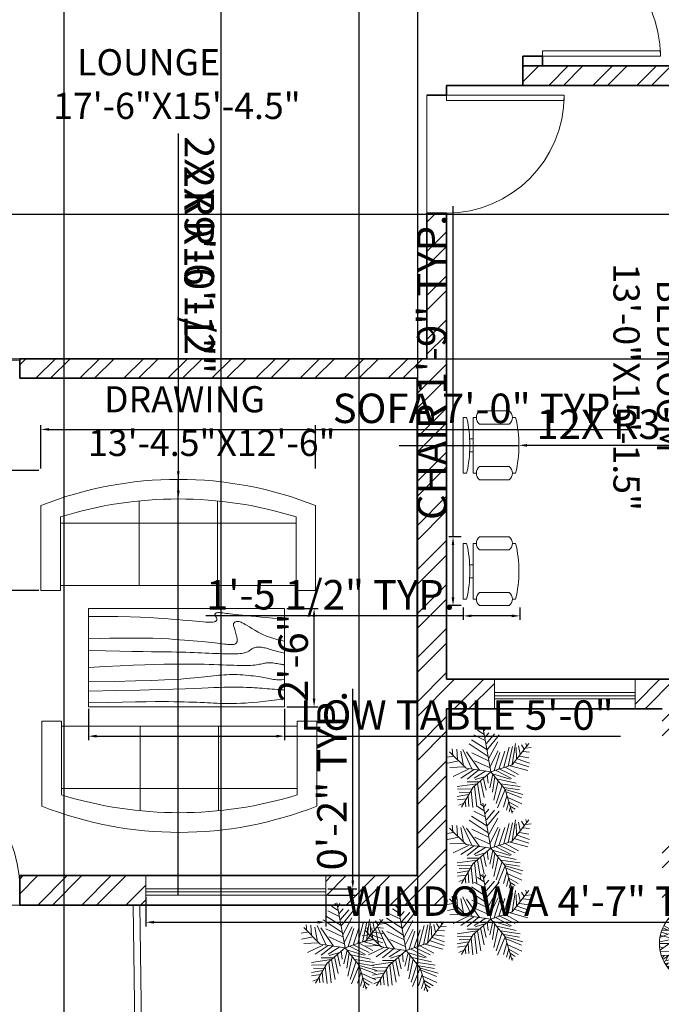
# Model space of a CAD drawing. Units: inches. Extents: x 744 to 1448, y 5126 to 6077.
# Tile 3 of 10: x 1025 to 1221, y 5284 to 5585. Entities that reach past the tile are written whole.
import ezdxf

# ---------------------------------------------------------------- set-up
doc = ezdxf.new("R2010")
doc.units = ezdxf.units.IN
for name, color, linetype, lineweight in [('A-ANNO-DIMS', 2, 'Continuous', 18), ('A-AREA-IDEN', 7, 'Continuous', 18), ('A-DOOR', 4, 'Continuous', 18), ('A-FURN', 8, 'Continuous', 18), ('A-SITE-PVMT', 8, 'Continuous', 18), ('A-WALL', 7, 'Continuous', 35), ('A-WALL-PATT', 252, 'Continuous', 13), ('L-PLNT', 3, 'Continuous', 13)]:
    doc.layers.add(name, color=color, linetype=linetype, lineweight=lineweight)
doc.layers.add('A-GLAZ', color=244, linetype='Continuous', lineweight=18, true_color=0x991b1e)
doc.styles.get("Standard").update_dxf_attribs({"font": 'arial.ttf'})
doc.dimstyles.new('ISO-25', dxfattribs={"dimtxt": 9, "dimasz": 2.5, "dimexe": 1.25, "dimexo": 0.625, "dimtad": 1, "dimlunit": 3, "dimtxsty": 'Standard', "dimcen": 2.5, "dimadec": 0, "dimazin": 0, "dimtfac": 1, "dimtmove": 0, "dimatfit": 3, "dimfxl": 1, "dimarcsym": 0})

# ---------------------------------------------------------------- blocks, each defined once
blk = doc.blocks.new('*U2')
for p, q in [((0, 0), (0, -6)), ((40, 0), (40, -6))]:
    blk.add_line(p, q)
blk.add_lwpolyline([(0, 0), (0, 40), (1.75, 40), (1.75, 0)], close=True)
blk.add_arc((0, 0), 40, 0, 90)
blk = doc.blocks.new('*U5')
for p, q in [((0, 0), (0, 6)), ((40, 0), (40, 6))]:
    blk.add_line(p, q)
blk.add_lwpolyline([(0, 0), (0, -40), (1.75, -40), (1.75, 0)], close=True)
blk.add_arc((0, 0), 40, 270, 0)
blk = doc.blocks.new('*U3')
for p, q in [((-40, 0), (-40, 6)), ((0, 0), (0, 6))]:
    blk.add_line(p, q)
blk.add_lwpolyline([(0, 0), (0, -40), (-1.75, -40), (-1.75, 0)], close=True)
blk.add_arc((0, 0), 40, 180, 270)
blk = doc.blocks.new('*U10')
for p, q in [((-8.737, 47.138), (-17.069, 52.711)), ((-10.186, 53.64), (-13.084, 55.962)), ((0, 0), (-10.5, 57)), ((-9.099, 51.782), (-6.563, 55.962)), ((-5.114, 28.097), (-24.676, 40.636)), ((-7.288, 39.707), (-21.778, 46.673)), ((-7.65, 43.423), (-2.578, 49.46)), ((-5.839, 35.992), (4.667, 48.067)), ((-5.114, 27.632), (10.463, 46.673)), ((-2.941, 16.486), (8.652, 37.85)), ((-31.5, 4.5), (-52.5, 25.5)), ((-48.585, 21.131), (-49.309, 29.026)), ((-43.513, 28.561), (-42.427, 15.558)), ((-38.442, 26.239), (-34.819, 7.663)), ((-35.544, 28.097), (-24.314, 3.947)), ((-14.533, 2.09), (-30.834, 25.31)), ((-3.665, 19.273), (-27.574, 35.527)), ((-1.129, 6.734), (9.014, 26.704)), ((10.101, 3.483), (17.708, 26.239)), ((16.259, 5.805), (23.142, 31.348)), ((22.055, 7.198), (27.489, 32.277)), ((27, 9), (48, 36)), ((27.127, 9.056), (31.112, 35.992)), ((31.836, 30.883), (32.561, 16.486)), ((35.096, 32.741), (37.27, 22.524)), ((38.719, 34.134), (41.979, 28.561)), ((40.53, 25.775), (48.862, 24.846)), ((43.791, 29.954), (51.036, 30.883)), ((44.153, 36.456), (45.239, 32.741)), ((-47.498, 19.737), (-55.83, 18.344)), ((-40.615, 13.7), (-55.105, 10.913)), ((-24.314, 23.917), (-2.941, 13.7)), ((-20.691, 13.7), (-1.129, 4.876)), ((3.942, 1.625), (11.187, 24.381)), ((33.285, 16.486), (48.862, 10.913)), ((36.183, 19.737), (48.137, 17.88)), ((-33.37, 6.269), (-52.207, 5.34)), ((-28.299, 3.483), (-47.86, -5.805)), ((-21.416, 3.018), (-38.079, -8.128)), ((0, 0), (-31.5, 4.5)), ((-15.982, 2.09), (-30.11, -9.521)), ((0, 0), (-22.5, -19.5)), ((-6.563, 1.161), (-21.416, -8.128)), ((0, 0), (27, 9)), ((0, 0), (18, -22.5)), ((6.478, 1.625), (26.04, -8.592)), ((11.187, 3.483), (30.749, -5.805)), ((18.07, 5.805), (35.096, -3.483)), ((24.229, 7.663), (46.688, 1.625)), ((29.662, 12.307), (48.137, 6.269)), ((-6.563, -5.805), (-19.967, -9.985)), ((-13.446, -11.378), (-8.737, -32.741)), ((-9.461, -8.592), (-6.201, -23.453)), ((-4.752, -3.483), (-3.665, -14.629)), ((2.493, -3.019), (-1.491, -20.202)), ((1.769, -2.555), (24.229, -9.521)), ((5.029, -6.27), (2.131, -25.775)), ((9.014, -11.378), (3.58, -35.992)), ((7.565, -9.056), (32.198, -14.629)), ((-17.431, -15.094), (-42.789, -18.809)), ((-24.314, -21.596), (-42.427, -22.06)), ((-22.5, -19.5), (-37.5, -45)), ((-15.257, -12.772), (-30.11, -12.772)), ((-25.038, -23.918), (-22.865, -45.281)), ((-20.691, -18.345), (-17.793, -44.352)), ((-17.069, -15.094), (-12.721, -40.172)), ((14.085, -16.951), (6.478, -40.172)), ((18.07, -22.524), (8.289, -45.745)), ((12.274, -15.094), (36.907, -18.809)), ((16.259, -19.738), (36.183, -22.989)), ((18, -22.5), (27, -52.5)), ((18.433, -22.524), (40.53, -29.026)), ((-28.299, -29.026), (-42.789, -31.348)), ((-30.834, -34.135), (-42.427, -35.528)), ((-26.849, -26.24), (-40.253, -25.775)), ((-32.646, -36.921), (-31.921, -44.352)), ((-29.023, -30.884), (-27.936, -43.887)), ((20.244, -30.419), (15.897, -44.816)), ((19.157, -25.311), (38.719, -33.206)), ((21.331, -32.741), (39.081, -40.636)), ((-34.457, -39.708), (-40.978, -42.494)), ((22.78, -37.85), (19.519, -48.532)), ((22.78, -38.314), (34.372, -44.816)), ((24.591, -45.745), (23.142, -50.854)), ((24.591, -43.423), (30.749, -47.603)), ((26.764, -49.925), (28.213, -50.854))]:
    blk.add_line(p, q)
blk = doc.blocks.new('*U13')
for p, q in [((-37.0107, 47.0408), (-35.25, 35.5298)), ((-32.6092, 50.4264), (-23.2782, 23.5674)), ((-31.2008, 51.1035), (-0.2149, 20.1818)), ((-26.4472, 46.5894), (-26.2712, 53.8116)), ((-22.0458, 42.0753), (-16.5881, 57.6486)), ((-21.1656, 55.8436), (-0.0388, 45.0094)), ((-12.5388, 54.9406), (-7.9613, 59.4546)), ((-12.3627, 32.1443), (-12.5388, 58.7776)), ((-5.3205, 59.6806), (16.5105, 16.7963)), ((2.426, 54.9406), (-1.4472, 59.9056)), ((0, 59.9996), (0, -60)), ((0.4894, 48.6208), (3.6584, 59.6806)), ((18.2711, 35.5298), (5.419, 59.6806)), ((9.8203, 51.5549), (12.8133, 58.5516)), ((19.6795, 19.5047), (16.3344, 57.6486)), ((17.0387, 51.1035), (23.2006, 55.1666)), ((17.7429, 43.6552), (25.4894, 54.2636)), ((31.6513, 50.8778), (30.2429, 30.5643)), ((31.1232, 42.5267), (35.8767, 48.1693)), ((-49.8627, 32.8214), (-32.7853, 32.8214)), ((-45.8134, 38.2383), (-40.5318, 33.0471)), ((-43.8768, 36.4326), (-44.405, 40.2696)), ((42, 42), (-42, -42)), ((42, -42), (-42, 42)), ((-40.1797, 44.558), (-36.4825, 43.2038)), ((36.2288, 25.1474), (48.9049, 35.0784)), ((37.1091, 37.1098), (46.6161, 37.5612)), ((-32.2571, 20.6333), (-59.1937, 9.348)), ((-57.081, 17.9248), (-47.0458, 14.7649)), ((-56.0247, 20.859), (-20.8134, 20.859)), ((-54.7923, 24.4702), (-47.75, 21.0847)), ((-53.2078, 27.4044), (-40.1797, 20.859)), ((54.3626, 25.3731), (20.9119, 0.3198)), ((23.3767, 23.3417), (53.3063, 27.4044)), ((-59.7219, 2.8025), (-12.0106, 12.0565)), ((-58.6656, 12.7336), (-35.9543, 7.5424)), ((-54.6162, -24.7335), (-20.2853, 0.0941)), ((29.3626, -6.6771), (59.4682, 7.091)), ((38.5175, 13.4107), (58.2359, 13.6364)), ((-60, 0), (60, 0)), ((-59.7219, -4.8714), (-54.2641, -6.6771)), ((-45.2853, -0.1316), (-59.0177, -10.0627)), ((-58.4895, -12.3197), (-36.4825, -11.6426)), ((-14.8275, -15.0282), (-14.6515, -57.6865)), ((-10.074, -10.0627), (-2.5036, -59.7178)), ((9.2922, -9.1598), (59.6443, -2.8401)), ((26.3697, -18.4138), (58.9401, -9.8369)), ((-57.081, -18.4138), (-45.2853, -17.9624)), ((-52.6797, -18.188), (-55.4966, -22.0251)), ((-53.2078, -27.442), (-16.7641, -16.6081)), ((-38.9472, -29.0219), (-51.4472, -30.6018)), ((-47.2219, -19.3166), (-50.2148, -26.3135)), ((-46.5177, -30.1504), (-49.5106, -33.536)), ((-35.9543, -22.4765), (-44.0529, -40.5329)), ((-19.9331, -20.2194), (-28.5599, -52.721)), ((-0.0388, -19.0909), (25.8415, -53.8495)), ((18.6232, -18.6394), (26.7218, -53.3981)), ((18.7992, -18.6394), (57.3556, -17.2853)), ((30.419, -30.1504), (32.3556, -50.0125)), ((38.1654, -18.188), (52.426, -29.0219)), ((45.9119, -24.0564), (55.595, -22.2508)), ((-32.4331, -32.4075), (-48.1021, -35.5674)), ((-43.7008, -34.6645), (-46.6937, -37.373)), ((-24.6867, -37.8244), (-38.7712, -45.7241)), ((-26.2712, -43.9185), (-34.7219, -48.6583)), ((-14.6515, -36.2445), (-27.6797, -52.9467)), ((-21.5177, -45.4984), (-19.9331, -56.1065)), ((-14.6515, -32.1818), (-3.912, -59.4922)), ((-6.2008, -36.2445), (17.919, -57.0094)), ((22.8485, -36.4702), (35.3485, -48.4326)), ((24.7852, -44.8213), (23.0246, -54.978)), ((31.4753, -31.279), (49.6091, -33.3103)), ((41.5105, -32.6332), (46.088, -38.0501)), ((-14.6515, -47.3041), (-25.0388, -54.3009)), ((-8.4895, -47.5298), (-11.4825, -58.5893)), ((-6.3768, -52.721), (-9.3698, -58.815)), ((8.4119, -53.1724), (3.8344, -59.4922)), ((5.9471, -46.6269), (10.5246, -58.5893))]:
    blk.add_line(p, q)
blk.add_circle((0, 0), 60)
blk = doc.blocks.new('Table - Rectangular Woodgrain 60 x 30 in.')
for p, q in [((0, 0), (0, -30)), ((60, 0), (0, 0)), ((60, -30), (60, 0)), ((0, -30), (60, -30))]:
    blk.add_line(p, q)
for points in [[(0, -2.4), (4.8155, -2.418), (9.0302, -2.4688), (12.709, -2.5477), (15.9167, -2.65), (18.7181, -2.7711), (21.1781, -2.9063), (23.3616, -3.0508), (25.3333, -3.2), (27.1477, -3.3495), (28.8172, -3.4958), (30.3437, -3.636), (31.7291, -3.7667), (32.9756, -3.8849), (34.0849, -3.9875), (35.059, -4.0714), (35.9, -4.1334), (36.6114, -4.1711), (37.2041, -4.1854), (37.6906, -4.1779), (38.0833, -4.15), (38.3948, -4.1034), (38.6375, -4.0396), (38.8239, -3.9602), (38.9666, -3.8667), (39.0764, -3.7608), (39.1573, -3.6448), (39.2116, -3.521), (39.2416, -3.3917), (39.2498, -3.2593), (39.2385, -3.1261), (39.21, -2.9944), (39.1666, -2.8667), (39.111, -2.7447), (39.0468, -2.6281), (38.978, -2.5163), (38.9083, -2.4083), (38.8418, -2.3035), (38.7823, -2.201), (38.7337, -2.1001), (38.7, -2), (38.6844, -1.9003), (38.6875, -1.8021), (38.7094, -1.707), (38.75, -1.6167), (38.8094, -1.5326), (38.8875, -1.4563), (38.9844, -1.3893), (39.1, -1.3333), (39.2351, -1.2896), (39.3937, -1.2583), (39.5804, -1.2396), (39.8, -1.2333), (40.057, -1.2396), (40.3562, -1.2583), (40.7023, -1.2896), (41.1, -1.3333), (41.5547, -1.3895), (42.0755, -1.4573), (42.6721, -1.5361), (43.3542, -1.625), (44.1316, -1.7233), (45.014, -1.8302), (46.0114, -1.9449), (47.1333, -2.0667), (48.3862, -2.1947), (49.7625, -2.3281), (51.2513, -2.4663), (52.8416, -2.6083), (54.5226, -2.7535), (56.2833, -2.9011), (58.1127, -3.0501), (60, -3.2)], [(0, -9.2), (6.5759, -9.0858), (11.9385, -9.0365), (16.2527, -9.0418), (19.6833, -9.0917), (22.3952, -9.1759), (24.5531, -9.2844), (26.322, -9.4069), (27.8666, -9.5333), (29.3241, -9.6553), (30.7203, -9.7719), (32.0532, -9.8837), (33.3208, -9.9917), (34.5213, -10.0965), (35.6526, -10.199), (36.7128, -10.2999), (37.7, -10.4), (38.6129, -10.4996), (39.4531, -10.5969), (40.223, -10.6895), (40.925, -10.775), (41.5613, -10.8512), (42.1344, -10.9156), (42.6465, -10.966), (43.1, -11), (43.4976, -11.0158), (43.8437, -11.0136), (44.143, -10.9942), (44.4, -10.9583), (44.6195, -10.9069), (44.8062, -10.8406), (44.9648, -10.7603), (45.1, -10.6667), (45.2155, -10.5598), (45.3114, -10.4365), (45.3871, -10.2929), (45.4416, -10.125), (45.4743, -9.929), (45.4844, -9.7011), (45.4709, -9.4371), (45.4333, -9.1333), (45.3716, -8.7883), (45.2896, -8.4104), (45.1919, -8.0107), (45.0833, -7.6), (44.9685, -7.1893), (44.8521, -6.7896), (44.7388, -6.4117), (44.6333, -6.0667), (44.54, -5.7628), (44.4614, -5.4979), (44.4001, -5.2675), (44.3583, -5.0667), (44.3384, -4.8909), (44.3427, -4.7354), (44.3736, -4.5956), (44.4333, -4.4667), (44.5236, -4.3453), (44.6427, -4.2333), (44.7884, -4.1339), (44.9583, -4.05), (45.1501, -3.9849), (45.3614, -3.9417), (45.59, -3.9234), (45.8333, -3.9333), (46.0915, -3.9749), (46.3734, -4.0531), (46.6906, -4.1736), (47.0542, -4.3417), (47.4756, -4.5629), (47.9661, -4.8427), (48.5372, -5.1866), (49.2, -5.6), (49.9676, -6.0844), (50.8594, -6.625), (51.8965, -7.2031), (53.1, -7.8), (54.491, -8.3969), (56.0906, -8.975), (57.9199, -9.5156), (60, -10)], [(0, -12.8), (5.1847, -12.9322), (9.6213, -13.0323), (13.3963, -13.1059), (16.5958, -13.1583), (19.3063, -13.1952), (21.614, -13.2219), (23.6054, -13.2439), (25.3666, -13.2667), (26.9728, -13.2947), (28.4531, -13.3281), (29.8256, -13.3663), (31.1083, -13.4083), (32.3191, -13.4535), (33.476, -13.501), (34.597, -13.5501), (35.7, -13.6), (36.7984, -13.6497), (37.8875, -13.6979), (38.9578, -13.743), (40, -13.7833), (41.0047, -13.8174), (41.9625, -13.8438), (42.864, -13.8607), (43.7, -13.8667), (44.4631, -13.8604), (45.1552, -13.8417), (45.7801, -13.8104), (46.3416, -13.7667), (46.8439, -13.7104), (47.2906, -13.6417), (47.6858, -13.5604), (48.0333, -13.4667), (48.3375, -13.3608), (48.6042, -13.2448), (48.8396, -13.121), (49.05, -12.9917), (49.2417, -12.8593), (49.4208, -12.7261), (49.5937, -12.5944), (49.7667, -12.4667), (49.9452, -12.3451), (50.1323, -12.2313), (50.3303, -12.1268), (50.5416, -12.0333), (50.7686, -11.9524), (51.0135, -11.8854), (51.2788, -11.8341), (51.5666, -11.8), (51.8785, -11.7843), (52.2116, -11.7865), (52.562, -11.8059), (52.926, -11.8417), (53.2998, -11.8931), (53.6795, -11.9594), (54.0614, -12.0397), (54.4416, -12.1333), (54.8223, -12.2401), (55.2293, -12.3625), (55.6942, -12.5037), (56.2489, -12.6667), (56.9251, -12.8547), (57.7545, -13.0708), (58.7689, -13.3182), (60, -13.6)], [(0, -18), (5.124, -17.7273), (9.6609, -17.5057), (13.6705, -17.3303), (17.2125, -17.1958), (20.3467, -17.0973), (23.1328, -17.0297), (25.6307, -16.9878), (27.9, -16.9667), (29.9928, -16.9617), (31.9302, -16.9703), (33.7254, -16.9907), (35.3917, -17.0208), (36.9423, -17.0588), (38.3906, -17.1026), (39.7499, -17.1503), (41.0333, -17.2), (42.2519, -17.2496), (43.4073, -17.2969), (44.4986, -17.3395), (45.525, -17.375), (46.4858, -17.4012), (47.3802, -17.4156), (48.2074, -17.416), (48.9667, -17.4), (49.6583, -17.3662), (50.2872, -17.3167), (50.8595, -17.2547), (51.3812, -17.1833), (51.8584, -17.1057), (52.2971, -17.025), (52.7034, -16.9443), (53.0833, -16.8667), (53.443, -16.7951), (53.789, -16.7313), (54.128, -16.6768), (54.4666, -16.6334), (54.8115, -16.6024), (55.1693, -16.5854), (55.5465, -16.5841), (55.95, -16.6), (56.3828, -16.6337), (56.8346, -16.6823), (57.2915, -16.7418), (57.7396, -16.8084), (58.165, -16.878), (58.5539, -16.9469), (58.8924, -17.0111), (59.1666, -17.0667), (59.3679, -17.1107), (59.5078, -17.1438), (59.6032, -17.1675), (59.6708, -17.1833), (59.7275, -17.193), (59.7901, -17.1979), (59.8753, -17.1998), (60, -17.2)], [(0, -22.4), (8.0098, -22.2501), (14.4094, -22.1011), (19.4168, -21.9535), (23.25, -21.8083), (26.1269, -21.6663), (28.2656, -21.5281), (29.884, -21.3947), (31.2, -21.2667), (32.3967, -21.1448), (33.5172, -21.0292), (34.5697, -20.9198), (35.5625, -20.8167), (36.5037, -20.7198), (37.4015, -20.6292), (38.2642, -20.5448), (39.1, -20.4667), (39.9164, -20.3951), (40.7187, -20.3313), (41.5117, -20.2768), (42.3, -20.2333), (43.0883, -20.2024), (43.8812, -20.1854), (44.6836, -20.1841), (45.5, -20.2), (46.3328, -20.234), (47.1747, -20.2844), (48.0163, -20.3488), (48.8479, -20.425), (49.66, -20.5106), (50.4429, -20.6031), (51.1872, -20.7004), (51.8833, -20.8), (52.5246, -20.8999), (53.1166, -20.9995), (53.6681, -21.0983), (54.1875, -21.1958), (54.6834, -21.2919), (55.1646, -21.3859), (55.6394, -21.4777), (56.1167, -21.5667), (56.6028, -21.6515), (57.0961, -21.7266), (57.5929, -21.7852), (58.0896, -21.8208), (58.5823, -21.8268), (59.0674, -21.7964), (59.5412, -21.723), (60, -21.6)], [(0, -25.2), (8.6355, -25.0504), (15.7026, -24.9031), (21.4049, -24.7606), (25.9458, -24.625), (29.529, -24.4988), (32.3578, -24.3844), (34.6359, -24.284), (36.5667, -24.2), (38.3213, -24.1341), (39.9417, -24.0854), (41.437, -24.0523), (42.8167, -24.0333), (44.0901, -24.0268), (45.2667, -24.0313), (46.3557, -24.0451), (47.3667, -24.0667), (48.309, -24.0947), (49.1928, -24.1287), (50.0284, -24.168), (50.826, -24.2125), (51.5959, -24.2617), (52.3483, -24.3151), (53.0935, -24.3725), (53.8417, -24.4334), (54.6009, -24.497), (55.3699, -24.561), (56.1454, -24.6226), (56.9239, -24.6792), (57.7021, -24.7279), (58.4764, -24.7662), (59.2435, -24.7911), (60, -24.8)], [(0, -28.8), (5.6867, -28.6681), (10.45, -28.5698), (14.407, -28.5012), (17.675, -28.4584), (20.3711, -28.4374), (22.6125, -28.4344), (24.5164, -28.4455), (26.2, -28.4667), (27.762, -28.4947), (29.2276, -28.5281), (30.6033, -28.5663), (31.8958, -28.6084), (33.1118, -28.6535), (34.2578, -28.7011), (35.3405, -28.7501), (36.3666, -28.8), (37.3443, -28.8497), (38.288, -28.8974), (39.2137, -28.9412), (40.1375, -28.9792), (41.0753, -29.0093), (42.0432, -29.0297), (43.0572, -29.0384), (44.1333, -29.0333), (45.2936, -29.0114), (46.5843, -28.9641), (48.0579, -28.8816), (49.7666, -28.7542), (51.7629, -28.5721), (54.0989, -28.3255), (56.8272, -28.0048), (60, -27.6)]]:
    blk.add_lwpolyline(points)
blk = doc.blocks.new('Sofa - Roundback 7 ft.')
for p, q in [((-12.00002, -32.4421), (-12.00003, -6.5971)), ((11.99997, -32.4421), (11.99998, -6.5971)), ((-36.000027, -34), (-36.000027, -11.4696)), ((35.99998, -34), (35.99998, -11.4696)), ((-35.999844, -13.3819), (35.9998, -13.3819)), ((-36.000027, -32.4421), (35.99998, -32.4421))]:
    blk.add_line(p, q)
for points in [[(-36.000027, -34), (-42.000027, -34), (-42.000027, -8)], [(41.99998, -8), (41.99998, -34), (35.99998, -34)]]:
    blk.add_lwpolyline(points)
for centre, radius, start, end in [((0, -114.25), 114.25, 68.43141, 111.5686), ((-0.00001, -127.1968), 121.1968, 72.72033, 107.2797)]:
    blk.add_arc(centre, radius, start, end)
blk = doc.blocks.new('Chair - Desk')
for p, q in [((-8.5, 0), (-8.5, -1)), ((-8.5, 0), (8.5, 0)), ((8.5, 0), (8.5, -1)), ((-8.5, -3), (-8.5, -4)), ((-8.5, -3), (8.5, -3)), ((-2, -3), (-2, -1.9355)), ((2, -1.9576), (2, -3)), ((8.5, -3), (8.5, -4)), ((-10.5, -5), (-10.5, -14)), ((-6.5, -14), (-6.5, -5)), ((6.5, -5), (6.5, -14)), ((10.5, -14), (10.5, -5)), ((-8.5, -15), (-8.5, -16)), ((8.5, -15), (8.5, -16))]:
    blk.add_line(p, q)
for centre, radius, start, end in [((0, 34.625), 36.625, 256.5803, 283.4197), ((-8.5, -6.5), 2.5, 36.8699, 143.1301), ((8.5, -6.5), 2.5, 36.8699, 143.1301), ((-8.5, -12.5), 2.5, 216.8699, 323.1301), ((8.5, -12.5), 2.5, 216.8699, 323.1301), ((0, 19.625), 36.625, 256.5803, 283.4197)]:
    blk.add_arc(centre, radius, start, end)
blk = doc.blocks.new('WINDOW-GLASS-55IN')
for p, q in [((0, 2), (55, 2)), ((0, 1), (55, 1)), ((0, 0), (55, 0))]:
    blk.add_line(p, q)
blk = doc.blocks.new('WINDOW-GLASS-43IN')
for p, q in [((0, 2), (43, 2)), ((0, 1), (43, 1)), ((0, 0), (43, 0))]:
    blk.add_line(p, q)
blk = doc.blocks.new('*D33')
at = {"layer": 'A-ANNO-DIMS', "color": 0, "lineweight": -2, "transparency": 16777216}
for p, q in [((1157.69, 5426.86), (1157.69, 5527.98)), ((1160.21, 5426.86), (1156.44, 5426.86)), ((1157.69, 5408.36), (1157.69, 5424.36)), ((1160.21, 5405.86), (1156.44, 5405.86))]:
    blk.add_line(p, q, dxfattribs=at)
at = {"layer": 'A-ANNO-DIMS', "color": 0, "transparency": 16777216}
for points in [[(1157.27, 5424.36), (1158.1, 5424.36), (1157.69, 5426.86)], [(1157.27, 5408.36), (1158.1, 5408.36), (1157.69, 5405.86)]]:
    blk.add_solid(points, dxfattribs=at)
at = {"layer": 'Defpoints', "color": 0, "transparency": 16777216}
for p in [(1157.69, 5426.86), (1160.84, 5426.86), (1160.84, 5405.86)]:
    blk.add_point(p, dxfattribs=at)
at = {"layer": 'A-ANNO-DIMS', "color": 0, "transparency": 16777216, "insert": (1152.41, 5478.67), "char_height": 9, "attachment_point": 5, "rotation": 90}
blk.add_mtext('CHAIR 1\'-9" TYP.', dxfattribs=at)
blk = doc.blocks.new('*D34')
at = {"layer": 'A-ANNO-DIMS', "color": 0, "lineweight": -2, "transparency": 16777216}
for p, q in [((1160.84, 5405.23), (1160.84, 5401.46)), ((1178.17, 5405.23), (1178.17, 5401.46)), ((1160.84, 5402.71), (1082.1, 5402.71)), ((1175.67, 5402.71), (1163.34, 5402.71))]:
    blk.add_line(p, q, dxfattribs=at)
at = {"layer": 'A-ANNO-DIMS', "color": 0, "transparency": 16777216}
for points in [[(1163.34, 5403.13), (1163.34, 5402.29), (1160.84, 5402.71)], [(1175.67, 5403.13), (1175.67, 5402.29), (1178.17, 5402.71)]]:
    blk.add_solid(points, dxfattribs=at)
at = {"layer": 'Defpoints', "color": 0, "transparency": 16777216}
for p in [(1160.84, 5405.86), (1178.17, 5405.86), (1160.84, 5402.71)]:
    blk.add_point(p, dxfattribs=at)
at = {"layer": 'A-ANNO-DIMS', "color": 0, "transparency": 16777216, "insert": (1120.22, 5407.99), "char_height": 9, "attachment_point": 5}
blk.add_mtext('1\'-5 1/2" TYP.', dxfattribs=at)
blk = doc.blocks.new('*D37')
at = {"layer": 'A-ANNO-DIMS', "color": 0, "lineweight": -2, "transparency": 16777216}
for p, q in [((1063.79, 5316.69), (1063.79, 5307.82)), ((1118.79, 5316.69), (1118.79, 5307.82)), ((1066.29, 5309.07), (1116.29, 5309.07)), ((1118.79, 5309.07), (1248.3, 5309.07))]:
    blk.add_line(p, q, dxfattribs=at)
at = {"layer": 'A-ANNO-DIMS', "color": 0, "transparency": 16777216}
for points in [[(1066.29, 5309.48), (1066.29, 5308.65), (1063.79, 5309.07)], [(1116.29, 5309.48), (1116.29, 5308.65), (1118.79, 5309.07)]]:
    blk.add_solid(points, dxfattribs=at)
at = {"layer": 'Defpoints', "color": 0, "transparency": 16777216}
for p in [(1063.79, 5317.32), (1118.79, 5317.32), (1118.79, 5309.07)]:
    blk.add_point(p, dxfattribs=at)
at = {"layer": 'A-ANNO-DIMS', "color": 0, "transparency": 16777216, "insert": (1184.8, 5314.35), "char_height": 9, "attachment_point": 5}
blk.add_mtext('WINDOW A 4\'-7" TYP.', dxfattribs=at)
blk = doc.blocks.new('*D38')
at = {"layer": 'A-ANNO-DIMS', "color": 0, "lineweight": -2, "transparency": 16777216}
for p, q in [((1127.04, 5321.82), (1127.04, 5380.43)), ((1119.41, 5319.32), (1128.29, 5319.32)), ((1127.04, 5317.32), (1127.04, 5319.32)), ((1119.41, 5317.32), (1128.29, 5317.32)), ((1127.04, 5314.82), (1127.04, 5312.32))]:
    blk.add_line(p, q, dxfattribs=at)
at = {"layer": 'A-ANNO-DIMS', "color": 0, "transparency": 16777216}
for points in [[(1126.62, 5321.82), (1127.45, 5321.82), (1127.04, 5319.32)], [(1126.62, 5314.82), (1127.45, 5314.82), (1127.04, 5317.32)]]:
    blk.add_solid(points, dxfattribs=at)
at = {"layer": 'Defpoints', "color": 0, "transparency": 16777216}
for p in [(1118.79, 5319.32), (1127.04, 5319.32), (1118.79, 5317.32)]:
    blk.add_point(p, dxfattribs=at)
at = {"layer": 'A-ANNO-DIMS', "color": 0, "transparency": 16777216, "insert": (1121.82, 5352.37), "char_height": 9, "attachment_point": 5, "rotation": 90}
blk.add_mtext('0\'-2" TYP.', dxfattribs=at)
blk = doc.blocks.new('*D43')
at = {"layer": 'A-ANNO-DIMS', "color": 0, "lineweight": -2, "transparency": 16777216}
for p, q in [((1031.68, 5447.73), (1031.68, 5460.95)), ((1034.18, 5459.7), (1113.18, 5459.7)), ((1115.68, 5447.73), (1115.68, 5460.95)), ((1115.68, 5459.7), (1211.97, 5459.7))]:
    blk.add_line(p, q, dxfattribs=at)
at = {"layer": 'A-ANNO-DIMS', "color": 0, "transparency": 16777216}
for points in [[(1034.18, 5460.12), (1034.18, 5459.29), (1031.68, 5459.7)], [(1113.18, 5460.12), (1113.18, 5459.29), (1115.68, 5459.7)]]:
    blk.add_solid(points, dxfattribs=at)
at = {"layer": 'Defpoints', "color": 0, "transparency": 16777216}
for p in [(1115.68, 5459.7), (1031.68, 5447.1), (1115.68, 5447.1)]:
    blk.add_point(p, dxfattribs=at)
at = {"layer": 'A-ANNO-DIMS', "color": 0, "transparency": 16777216, "insert": (1165.08, 5464.98), "char_height": 9, "attachment_point": 5}
blk.add_mtext('SOFA 7\'-0" TYP.', dxfattribs=at)
blk = doc.blocks.new('*D44')
at = {"layer": 'A-ANNO-DIMS', "color": 0, "lineweight": -2, "transparency": 16777216}
for p, q in [((1019.08, 5447.1), (1019.08, 5526.68)), ((1031.06, 5447.1), (1017.83, 5447.1)), ((1019.08, 5412.94), (1019.08, 5444.6)), ((1031.06, 5410.44), (1017.83, 5410.44))]:
    blk.add_line(p, q, dxfattribs=at)
at = {"layer": 'A-ANNO-DIMS', "color": 0, "transparency": 16777216}
for points in [[(1018.66, 5444.6), (1019.5, 5444.6), (1019.08, 5447.1)], [(1018.66, 5412.94), (1019.5, 5412.94), (1019.08, 5410.44)]]:
    blk.add_solid(points, dxfattribs=at)
at = {"layer": 'Defpoints', "color": 0, "transparency": 16777216}
for p in [(1019.08, 5447.1), (1031.68, 5447.1), (1031.68, 5410.44)]:
    blk.add_point(p, dxfattribs=at)
at = {"layer": 'A-ANNO-DIMS', "color": 0, "transparency": 16777216, "insert": (1013.8, 5488.14), "char_height": 9, "attachment_point": 5, "rotation": 90}
blk.add_mtext('3\'-0 1/2" TYP.', dxfattribs=at)
blk = doc.blocks.new('*D45')
at = {"layer": 'A-ANNO-DIMS', "color": 0, "lineweight": -2, "transparency": 16777216}
for p, q in [((1046.21, 5374.32), (1046.21, 5364.69)), ((1106.21, 5374.32), (1106.21, 5364.69)), ((1048.71, 5365.94), (1103.71, 5365.94)), ((1106.21, 5365.94), (1208.94, 5365.94))]:
    blk.add_line(p, q, dxfattribs=at)
at = {"layer": 'A-ANNO-DIMS', "color": 0, "transparency": 16777216}
for points in [[(1048.71, 5366.36), (1048.71, 5365.53), (1046.21, 5365.94)], [(1103.71, 5366.36), (1103.71, 5365.53), (1106.21, 5365.94)]]:
    blk.add_solid(points, dxfattribs=at)
at = {"layer": 'Defpoints', "color": 0, "transparency": 16777216}
for p in [(1046.21, 5374.94), (1106.21, 5374.94), (1106.21, 5365.94)]:
    blk.add_point(p, dxfattribs=at)
at = {"layer": 'A-ANNO-DIMS', "color": 0, "transparency": 16777216, "insert": (1158.83, 5371.23), "char_height": 9, "attachment_point": 5}
blk.add_mtext('LOW TABLE 5\'-0"', dxfattribs=at)
blk = doc.blocks.new('*D46')
at = {"layer": 'A-ANNO-DIMS', "color": 0, "lineweight": -2, "transparency": 16777216}
for p, q in [((1106.83, 5404.94), (1116.46, 5404.94)), ((1115.21, 5377.44), (1115.21, 5402.44)), ((1106.83, 5374.94), (1116.46, 5374.94))]:
    blk.add_line(p, q, dxfattribs=at)
at = {"layer": 'A-ANNO-DIMS', "color": 0, "transparency": 16777216}
for points in [[(1114.79, 5402.44), (1115.63, 5402.44), (1115.21, 5404.94)], [(1114.79, 5377.44), (1115.63, 5377.44), (1115.21, 5374.94)]]:
    blk.add_solid(points, dxfattribs=at)
at = {"layer": 'Defpoints', "color": 0, "transparency": 16777216}
for p in [(1106.21, 5404.94), (1115.21, 5404.94), (1106.21, 5374.94)]:
    blk.add_point(p, dxfattribs=at)
at = {"layer": 'A-ANNO-DIMS', "color": 0, "transparency": 16777216, "insert": (1109.99, 5389.94), "char_height": 9, "attachment_point": 5, "rotation": 90}
blk.add_mtext('2\'-6"', dxfattribs=at)
blk = doc.blocks.new('*D56')
at = {"layer": 'A-ANNO-DIMS', "color": 0, "lineweight": -2, "transparency": 16777216}
for p, q in [((1038.68, 5750.19), (1038.68, 5125.91)), ((1086.68, 5750.19), (1086.68, 5125.91)), ((1041.18, 5127.16), (1084.18, 5127.16))]:
    blk.add_line(p, q, dxfattribs=at)
at = {"layer": 'A-ANNO-DIMS', "color": 0, "transparency": 16777216}
for points in [[(1041.18, 5127.58), (1041.18, 5126.75), (1038.68, 5127.16)], [(1084.18, 5127.58), (1084.18, 5126.75), (1086.68, 5127.16)]]:
    blk.add_solid(points, dxfattribs=at)
at = {"layer": 'Defpoints', "color": 0, "transparency": 16777216}
for p in [(1038.68, 5750.82), (1086.68, 5750.82), (1086.68, 5127.16)]:
    blk.add_point(p, dxfattribs=at)
at = {"layer": 'A-ANNO-DIMS', "color": 0, "transparency": 16777216, "insert": (1062.68, 5132.38), "char_height": 9, "attachment_point": 5}
blk.add_mtext('4\'-0"', dxfattribs=at)
blk = doc.blocks.new('*D58')
at = {"layer": 'A-ANNO-DIMS', "color": 0, "lineweight": -2, "transparency": 16777216}
for p, q in [((1128.86, 5714.27), (1128.86, 5125.91)), ((1146.83, 5714.27), (1146.83, 5125.91)), ((1131.36, 5127.16), (1144.33, 5127.16)), ((1146.83, 5127.16), (1173.66, 5127.16))]:
    blk.add_line(p, q, dxfattribs=at)
at = {"layer": 'A-ANNO-DIMS', "color": 0, "transparency": 16777216}
for points in [[(1131.36, 5127.58), (1131.36, 5126.75), (1128.86, 5127.16)], [(1144.33, 5127.58), (1144.33, 5126.75), (1146.83, 5127.16)]]:
    blk.add_solid(points, dxfattribs=at)
at = {"layer": 'Defpoints', "color": 0, "transparency": 16777216}
for p in [(1128.86, 5714.9), (1146.83, 5714.9), (1146.83, 5127.16)]:
    blk.add_point(p, dxfattribs=at)
at = {"layer": 'A-ANNO-DIMS', "color": 0, "transparency": 16777216, "insert": (1161.49, 5132.38), "char_height": 9, "attachment_point": 5}
blk.add_mtext('1\'-6"', dxfattribs=at)
blk = doc.blocks.new('*D61')
at = {"layer": 'A-ANNO-DIMS', "color": 0, "lineweight": -2, "transparency": 16777216}
for p, q in [((905.31, 5525.47), (1415.33, 5525.47)), ((1414.08, 5483.82), (1414.08, 5522.97)), ((905.31, 5481.32), (1415.33, 5481.32))]:
    blk.add_line(p, q, dxfattribs=at)
at = {"layer": 'A-ANNO-DIMS', "color": 0, "transparency": 16777216}
for points in [[(1413.67, 5522.97), (1414.5, 5522.97), (1414.08, 5525.47)], [(1413.67, 5483.82), (1414.5, 5483.82), (1414.08, 5481.32)]]:
    blk.add_solid(points, dxfattribs=at)
at = {"layer": 'Defpoints', "color": 0, "transparency": 16777216}
for p in [(904.68, 5525.47), (1414.08, 5525.47), (904.68, 5481.32)]:
    blk.add_point(p, dxfattribs=at)
at = {"layer": 'A-ANNO-DIMS', "color": 0, "transparency": 16777216, "insert": (1408.86, 5503.39), "char_height": 9, "attachment_point": 5, "rotation": 90}
blk.add_mtext('3\'-8"', dxfattribs=at)
blk = doc.blocks.new('*D63')
at = {"layer": 'A-ANNO-DIMS', "color": 0, "lineweight": -2, "transparency": 16777216}
for p, q in [((1073.68, 5541.29), (1073.68, 5440.94)), ((1073.68, 5317.24), (1073.68, 5438.44))]:
    blk.add_line(p, q, dxfattribs=at)
at = {"layer": 'A-ANNO-DIMS', "color": 0, "transparency": 16777216}
blk.add_solid([(1074.1, 5440.94), (1073.26, 5440.94), (1073.68, 5438.44)], dxfattribs=at)
at = {"layer": 'Defpoints', "color": 0, "transparency": 16777216}
for p in [(1073.68, 5438.44), (1073.68, 5317.24)]:
    blk.add_point(p, dxfattribs=at)
at = {"layer": 'A-ANNO-DIMS', "color": 0, "transparency": 16777216, "insert": (1078.9, 5511.15), "char_height": 9, "attachment_point": 5, "rotation": 270.0002}
blk.add_mtext('2X R10\'-1"', dxfattribs=at)
blk = doc.blocks.new('*D64')
at = {"layer": 'A-ANNO-DIMS', "color": 0, "lineweight": -2, "transparency": 16777216}
for p, q in [((1073.68, 5550.11), (1073.68, 5446.94)), ((1073.68, 5330.19), (1073.68, 5444.44))]:
    blk.add_line(p, q, dxfattribs=at)
at = {"layer": 'A-ANNO-DIMS', "color": 0, "transparency": 16777216}
blk.add_solid([(1074.1, 5446.94), (1073.26, 5446.94), (1073.68, 5444.44)], dxfattribs=at)
at = {"layer": 'Defpoints', "color": 0, "transparency": 16777216}
for p in [(1073.68, 5444.44), (1073.68, 5330.19)]:
    blk.add_point(p, dxfattribs=at)
at = {"layer": 'A-ANNO-DIMS', "color": 0, "transparency": 16777216, "insert": (1078.96, 5512.99), "char_height": 9, "attachment_point": 5, "rotation": 270.0002}
blk.add_mtext('2X R9\'-6 1/2"', dxfattribs=at)
blk = doc.blocks.new('*D65')
at = {"layer": 'A-ANNO-DIMS', "color": 0, "lineweight": -2, "transparency": 16777216}
for p, q in [((1141.21, 5454.83), (1177.84, 5454.83)), ((1263.08, 5454.83), (1180.34, 5454.83))]:
    blk.add_line(p, q, dxfattribs=at)
at = {"layer": 'A-ANNO-DIMS', "color": 0, "transparency": 16777216}
blk.add_solid([(1180.34, 5455.25), (1180.34, 5454.41), (1177.84, 5454.83)], dxfattribs=at)
at = {"layer": 'Defpoints', "color": 0, "transparency": 16777216}
for p in [(1141.21, 5454.83), (1177.84, 5454.83)]:
    blk.add_point(p, dxfattribs=at)
at = {"layer": 'A-ANNO-DIMS', "color": 0, "transparency": 16777216, "insert": (1222.96, 5460.11), "char_height": 9, "attachment_point": 5, "rotation": 0.0006}
blk.add_mtext('12X R3\'-0 1/2"', dxfattribs=at)

msp = doc.modelspace()

# ---------------------------------------------------------------- hatches: boundary and pattern name
at = {"layer": 'A-WALL-PATT'}
h = msp.add_hatch(dxfattribs=at)
h.set_pattern_fill('ANSI32', color=256)
h.paths.add_polyline_path([(813.684, 5750.816), (876.684, 5750.816), (876.684, 5756.816), (813.684, 5756.816), (813.684, 5812.816), (909.684, 5812.816), (909.684, 5795.316), (915.684, 5795.316), (915.684, 5812.816), (1209.684, 5812.816), (1209.684, 5795.316), (1215.684, 5795.316), (1215.684, 5812.816), (1311.684, 5812.816), (1311.684, 5756.816), (1248.684, 5756.816), (1248.684, 5750.816), (1311.684, 5750.816), (1311.684, 5570.816), (1179.044, 5570.816), (1179.044, 5564.816), (1311.684, 5564.816), (1311.684, 5383.316), (1260.684, 5383.316), (1260.684, 5377.316), (1311.684, 5377.316), (1311.684, 5320.316), (1227.684, 5320.316), (1227.684, 5333.816), (1221.684, 5333.816), (1221.684, 5314.316), (1320.684, 5314.316), (1320.684, 5821.816), (804.684, 5821.816), (804.684, 5472.316), (926.184, 5472.316), (926.184, 5481.316), (813.684, 5481.316), (813.684, 5581.616), (946.284, 5581.616), (946.284, 5587.616), (813.684, 5587.616)])
h.paths.add_polyline_path([(1155.684, 5525.816), (1149.684, 5525.816), (1149.684, 5481.316), (1025.184, 5481.316), (1025.184, 5475.316), (1146.684, 5475.316), (1146.684, 5323.316), (1118.788, 5323.316), (1118.788, 5314.316), (1146.684, 5314.316), (1155.684, 5314.316), (1155.684, 5374.316), (1170.35, 5374.316), (1170.35, 5383.316), (1155.684, 5383.316)], flags=17)
h.paths.add_polyline_path([(1230.684, 5383.316), (1213.35, 5383.316), (1213.35, 5374.316), (1221.684, 5374.316), (1221.684, 5363.816), (1226.184, 5363.816), (1227.684, 5363.816), (1227.684, 5377.316), (1230.684, 5377.316)], flags=17)
h.paths.add_polyline_path([(1185.684, 5671.816), (1155.684, 5671.816), (1155.684, 5750.816), (1161.575, 5750.816), (1161.575, 5756.816), (1157.542, 5756.816), (1157.847, 5756.715), (1155.79, 5756.816), (1149.684, 5756.816), (1149.684, 5750.816), (1149.684, 5671.816), (1121.684, 5671.816), (1121.684, 5665.816), (1179.684, 5665.816), (1179.684, 5609.816), (1185.684, 5609.816)], flags=17)
h.paths.add_polyline_path([(1003.684, 5671.816), (975.684, 5671.816), (975.684, 5750.816), (975.684, 5756.816), (965.205, 5756.816), (965.205, 5750.816), (969.684, 5750.816), (969.684, 5671.816), (939.684, 5671.816), (939.684, 5626.616), (945.684, 5626.616), (945.684, 5665.816), (1003.684, 5665.816)], flags=17)
h.paths.add_polyline_path([(915.684, 5774.316), (909.684, 5774.316), (909.684, 5756.816), (906.684, 5756.816), (906.684, 5752.316), (906.684, 5750.816), (922.205, 5750.816), (922.205, 5756.816), (915.684, 5756.816)], flags=17)
h.paths.add_polyline_path([(1215.684, 5774.316), (1209.684, 5774.316), (1209.684, 5756.816), (1204.575, 5756.816), (1204.575, 5750.816), (1218.684, 5750.816), (1218.684, 5756.816), (1215.684, 5756.816)], flags=17)
h.paths.add_polyline_path([(1063.788, 5323.316), (1025.184, 5323.316), (1025.184, 5314.316), (1063.788, 5314.316)])
h.paths.add_polyline_path([(986.184, 5475.316), (989.184, 5475.316), (989.184, 5481.316), (974.184, 5481.316), (974.184, 5475.916), (974.184, 5472.316), (977.184, 5472.316), (977.184, 5314.316), (989.184, 5314.316), (989.184, 5319.716), (989.184, 5323.316), (986.184, 5323.316)])

# ---------------------------------------------------------------- linework, layer by layer
at = {"layer": 'A-DOOR'}
for p, q in [((1149.684, 5525.816), (1149.684, 5561.816)), ((989.184, 5481.316), (1025.184, 5480.716)), ((1025.184, 5314.316), (989.184, 5314.316))]:
    msp.add_line(p, q, dxfattribs=at)
at = {"layer": 'A-GLAZ'}
for points in [[(1170.35, 5383.316), (1213.35, 5383.316), (1213.35, 5374.316), (1170.35, 5374.316)], [(1063.788, 5323.316), (1118.788, 5323.316), (1118.788, 5314.316), (1063.788, 5314.316)]]:
    msp.add_lwpolyline(points, close=True, dxfattribs=at)
at = {"layer": 'A-SITE-PVMT'}
for p, q in [((1059.934, 5314.29), (1060.684, 5256.29)), ((1061.934, 5314.316), (1062.684, 5256.316))]:
    msp.add_line(p, q, dxfattribs=at)
at = {"layer": 'A-WALL'}
for p, q in [((1185.044, 5573.816), (1179.044, 5573.816)), ((1179.044, 5573.816), (1179.044, 5564.816)), ((1185.044, 5570.816), (1185.044, 5573.816)), ((1179.044, 5570.816), (1311.684, 5570.816)), ((1155.684, 5564.816), (1311.684, 5564.816)), ((1155.684, 5561.816), (1155.684, 5564.816)), ((1155.684, 5561.816), (1149.684, 5561.816)), ((1149.684, 5481.316), (1149.684, 5525.816)), ((1155.684, 5525.816), (1149.684, 5525.816)), ((1155.684, 5383.316), (1155.684, 5525.816)), ((1025.184, 5475.316), (1025.184, 5481.316)), ((1025.184, 5481.316), (1149.684, 5481.316)), ((1025.184, 5475.316), (1146.684, 5475.316)), ((1146.684, 5323.316), (1146.684, 5475.316)), ((1155.684, 5383.316), (1311.684, 5383.316)), ((1155.684, 5314.316), (1155.684, 5374.316)), ((1155.684, 5374.316), (1221.684, 5374.316)), ((1025.184, 5323.316), (1025.184, 5314.316)), ((1025.184, 5323.316), (1146.684, 5323.316)), ((1025.184, 5314.316), (1146.684, 5314.316)), ((1146.684, 5314.316), (1155.684, 5314.316))]:
    msp.add_line(p, q, dxfattribs=at)

# ---------------------------------------------------------------- block references
at = {"layer": 'A-DOOR', "xscale": 0.9, "yscale": 0.9, "zscale": 0.9, "rotation": 90}
for name, p in [('*U5', (1185.084, 5573.816)), ('*U3', (1155.684, 5561.816))]:
    msp.add_blockref(name, p, dxfattribs=at)
at = {"layer": 'A-DOOR', "xscale": 0.9, "yscale": 0.9, "zscale": 0.9}
msp.add_blockref('*U2', (989.184, 5319.716), dxfattribs=at)
at = {"layer": 'A-FURN', "rotation": 90}
for p in [(1160.836, 5454.831), (1160.836, 5416.359)]:
    msp.add_blockref('Chair - Desk', p, dxfattribs=at)
at = {"layer": 'A-FURN'}
for name, p in [('Sofa - Roundback 7 ft.', (1073.68, 5444.436)), ('Table - Rectangular Woodgrain 60 x 30 in.', (1046.21, 5404.944))]:
    msp.add_blockref(name, p, dxfattribs=at)
at = {"layer": 'A-FURN', "xscale": -1, "rotation": 180}
msp.add_blockref('Sofa - Roundback 7 ft.', (1074.002, 5336.542), dxfattribs=at)
at = {"layer": 'A-GLAZ', "rotation": 180}
msp.add_blockref('WINDOW-GLASS-43IN', (1213.35, 5379.316), dxfattribs=at)
at = {"layer": 'A-GLAZ'}
msp.add_blockref('WINDOW-GLASS-55IN', (1063.788, 5317.316), dxfattribs=at)
at = {"layer": 'L-PLNT'}
for name, p, xscale, yscale, zscale in [('*U10', (1169.291, 5355.059), 0.2409161369388113, 0.2409161369388113, 0.2409161369388113), ('*U10', (1169.291, 5331.729), 0.2409161369388113, 0.2409161369388113, 0.2409161369388113), ('*U10', (1169.291, 5310.056), 0.2409161369388113, 0.2409161369388113, 0.2409161369388113), ('*U10', (1124.676, 5301.272), 0.2409161369388113, 0.2409161369388113, 0.2409161369388113), ('*U10', (1143.338, 5300.477), 0.2409161369388113, 0.2409161369388113, 0.2409161369388113), ('*U13', (1232.666, 5302.543), 0.1976487053468327, 0.1976487053468327, 0.1976487053468327)]:
    msp.add_blockref(name, p, dxfattribs=dict(at, xscale=xscale, yscale=yscale, zscale=zscale))

# ---------------------------------------------------------------- texts
at = {"layer": 'A-AREA-IDEN', "char_height": 8, "attachment_point": 1}
for s, insert in [('   LOUNGE\\P17\'-6"X15\'-4.5"', (1035.419, 5575.923)), ('  DRAWING\\P13\'-4.5"X12\'-6"', (1046.082, 5472.914))]:
    msp.add_mtext_dynamic_manual_height_columns(s, width=70.44947, gutter_width=12.5, heights=[0], dxfattribs=dict(at, insert=insert))
at = {"layer": 'A-AREA-IDEN', "insert": (1228.074, 5510.459), "char_height": 8, "attachment_point": 1, "rotation": 270}
msp.add_mtext_dynamic_manual_height_columns('  BEDROOM\\P13\'-0"X15\'-1.5"', width=73.67045, gutter_width=12.5, heights=[0], dxfattribs=at)

# ---------------------------------------------------------------- dimensions: what is measured, and where the dimension line sits
at = {"layer": 'A-ANNO-DIMS'}
for base, p1, p2, picture, middle in [((1086.684, 5127.162), (1038.684, 5750.816), (1086.684, 5750.816), '*D56', (1062.684, 5132.383)), ((1146.829, 5127.162), (1128.864, 5714.896), (1146.829, 5714.896), '*D58', (1161.493, 5132.383))]:
    dim = msp.add_linear_dim(base=base, p1=p1, p2=p2, dimstyle='ISO-25', override={"dimdec": 1, "dimlfac": 1, "dimrnd": 0, "dimzin": 1, "dimdsep": 46, "dimlunit": 4, "dimfrac": 2}, dxfattribs=at)
    dim.commit()
    dim.dimension.update_dxf_attribs({"geometry": picture, "text_midpoint": middle})
for center, mpoint, picture, middle in [((1073.680371, 5330.186), (1073.68, 5444.436), '*D64', (1073.6797774, 5512.986)), ((1073.68, 5317.239), (1073.68, 5438.436), '*D63', (1073.68, 5511.154))]:
    dim = msp.add_radius_dim(center=center, mpoint=mpoint, text='2X <>', dimstyle='ISO-25', override={"dimdec": 1, "dimlfac": 1, "dimrnd": 0, "dimzin": 1, "dimdsep": 46, "dimlunit": 4, "dimfrac": 2}, dxfattribs=at)
    dim.commit()
    dim.dimension.update_dxf_attribs({"geometry": picture, "text_midpoint": middle, "dimtype": 164})
for base, p1, p2, picture, middle in [((1414.084316, 5525.465662), (904.684316, 5481.315662), (904.684316, 5525.465662), '*D61', (1408.861089533, 5503.390662)), ((1115.21, 5404.944), (1106.21, 5374.944), (1106.21, 5404.944), '*D46', (1109.99, 5389.944))]:
    dim = msp.add_linear_dim(base=base, p1=p1, p2=p2, angle=90, dimstyle='ISO-25', override={"dimdec": 1, "dimlfac": 1, "dimrnd": 0, "dimzin": 1, "dimdsep": 46, "dimlunit": 4, "dimfrac": 2}, dxfattribs=at)
    dim.commit()
    dim.dimension.update_dxf_attribs({"geometry": picture, "text_midpoint": middle})
for base, p1, p2, angle, text, picture, middle in [((1019.08, 5447.103), (1031.68, 5410.436), (1031.68, 5447.103), 90, '<> TYP.', '*D44', (1013.799, 5488.14)), ((1157.686, 5426.859), (1160.836, 5405.859), (1160.836, 5426.859), 90, 'CHAIR <> TYP.', '*D33', (1152.408, 5478.668)), ((1160.836, 5402.709), (1178.17, 5405.859), (1160.836, 5405.859), 180, '<> TYP.', '*D34', (1120.219, 5407.988)), ((1127.038, 5319.316), (1118.788, 5317.316), (1118.788, 5319.316), 90, '<> TYP.', '*D38', (1121.818, 5352.37))]:
    dim = msp.add_linear_dim(base=base, p1=p1, p2=p2, angle=angle, text=text, dimstyle='ISO-25', override={"dimdec": 1, "dimlfac": 1, "dimrnd": 0, "dimzin": 1, "dimdsep": 46, "dimlunit": 4, "dimfrac": 2}, dxfattribs=at)
    dim.commit()
    dim.dimension.update_dxf_attribs({"geometry": picture, "text_midpoint": middle})
for base, p1, p2, text, picture, middle in [((1115.68, 5459.703), (1031.68, 5447.103), (1115.68, 5447.103), 'SOFA <> TYP.', '*D43', (1165.076, 5464.984)), ((1106.21, 5365.944), (1046.21, 5374.944), (1106.21, 5374.944), 'LOW TABLE <>', '*D45', (1158.826, 5371.225)), ((1118.788, 5309.066), (1063.788, 5317.316), (1118.788, 5317.316), 'WINDOW A <> TYP.', '*D37', (1184.796, 5314.347))]:
    dim = msp.add_linear_dim(base=base, p1=p1, p2=p2, text=text, dimstyle='ISO-25', override={"dimdec": 1, "dimlfac": 1, "dimrnd": 0, "dimzin": 1, "dimdsep": 46, "dimlunit": 4, "dimfrac": 2}, dxfattribs=at)
    dim.commit()
    dim.dimension.update_dxf_attribs({"geometry": picture, "text_midpoint": middle})
dim = msp.add_radius_dim(center=(1141.211, 5454.831), mpoint=(1177.836, 5454.831), text='12X <>', dimstyle='ISO-25', override={"dimdec": 1, "dimlfac": 1, "dimrnd": 0, "dimzin": 1, "dimdsep": 46, "dimlunit": 4, "dimfrac": 2}, dxfattribs=at)
dim.commit()
dim.dimension.update_dxf_attribs({"geometry": '*D65', "text_midpoint": (1222.958, 5460.113)})

doc.saveas('drawing.dxf')
